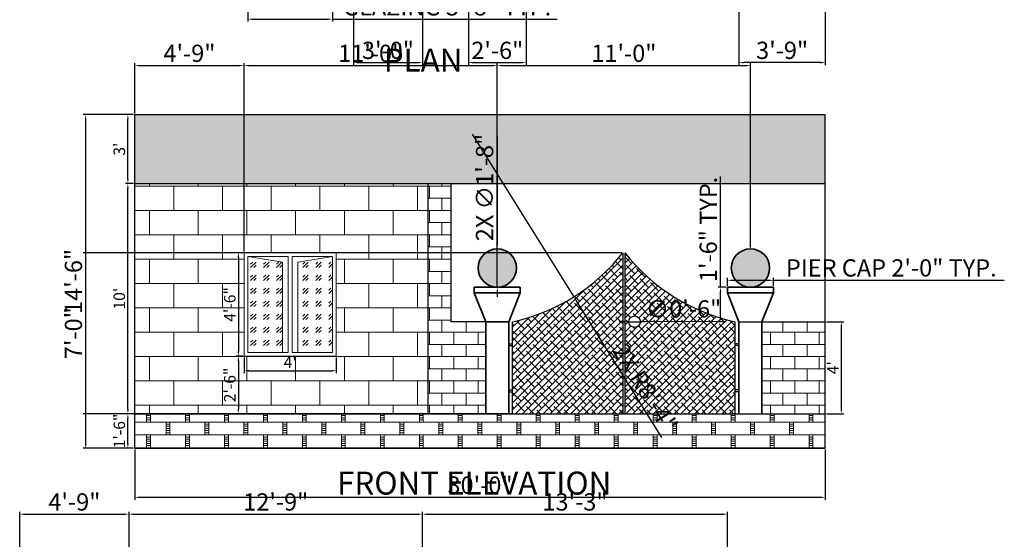
# Model space of a CAD drawing. Units: inches. Extents: x 2639 to 6021, y 292 to 2009.
# Tile 3 of 6: x 2676 to 3189, y 971 to 1243. Entities that reach past the tile are written whole.
import ezdxf

# ---------------------------------------------------------------- set-up
doc = ezdxf.new("R2010")
doc.units = ezdxf.units.IN
for name, color, linetype, lineweight in [('A-ANNO-DIMS', 2, 'Continuous', 18), ('A-ANNO-TEXT', 7, 'Continuous', 18), ('A-COLS', 7, 'Continuous', 35), ('A-DOOR-GATE', 3, 'Continuous', 25), ('A-ELEV', 7, 'Continuous', 30), ('A-ELEV-PATT', 8, 'Continuous', 13), ('A-GLAZ', 4, 'Continuous', 18), ('A-GLAZ-PATT', 9, 'Continuous', 13)]:
    doc.layers.add(name, color=color, linetype=linetype, lineweight=lineweight)
for name, color, linetype, lineweight, true_color in [('A-COLS-PATT', 251, 'Continuous', 13, 0x636466), ('A-DOOR-GATE-PATT', 251, 'Continuous', 13, 0x636466), ('A-ELEV-MASN-PATT', 30, 'Continuous', 13, 0xf26722)]:
    doc.layers.add(name, color=color, linetype=linetype, lineweight=lineweight, true_color=true_color)
doc.styles.get("Standard").update_dxf_attribs({"font": 'arial.ttf'})
doc.dimstyles.new('ISO-25', dxfattribs={"dimtxt": 9, "dimasz": 2.5, "dimexe": 1.25, "dimexo": 0.625, "dimtad": 1, "dimdec": 1, "dimlunit": 3, "dimtxsty": 'Standard', "dimcen": 2.5, "dimadec": 0, "dimazin": 0, "dimtfac": 1, "dimtdec": 1, "dimtmove": 0, "dimatfit": 3, "dimfxl": 1, "dimarcsym": 0})

# ---------------------------------------------------------------- blocks, each defined once
blk = doc.blocks.new('*D9')
at = {"layer": 'A-ANNO-DIMS', "color": 0, "lineweight": -2, "transparency": 16777216}
for p, q in [((2735.48, 1036.99), (2731.25, 1036.99)), ((2732.5, 1021.49), (2732.5, 1034.49)), ((2735.48, 1018.99), (2731.25, 1018.99))]:
    blk.add_line(p, q, dxfattribs=at)
at = {"layer": 'A-ANNO-DIMS', "color": 0, "transparency": 16777216}
for points in [[(2732.09, 1034.49), (2732.92, 1034.49), (2732.5, 1036.99)], [(2732.09, 1021.49), (2732.92, 1021.49), (2732.5, 1018.99)]]:
    blk.add_solid(points, dxfattribs=at)
at = {"layer": 'Defpoints', "color": 0, "transparency": 16777216}
for p in [(2732.5, 1036.99), (2736.11, 1036.99), (2736.11, 1018.99)]:
    blk.add_point(p, dxfattribs=at)
at = {"layer": 'A-ANNO-DIMS', "color": 0, "transparency": 16777216, "insert": (2728.81, 1027.99), "char_height": 6, "attachment_point": 5, "rotation": 90}
blk.add_mtext('1\'-6"', dxfattribs=at)
blk = doc.blocks.new('*D10')
at = {"layer": 'A-ANNO-DIMS', "color": 0, "lineweight": -2, "transparency": 16777216}
for p, q in [((2735.48, 1156.99), (2731.25, 1156.99)), ((2732.5, 1039.49), (2732.5, 1154.49)), ((2735.48, 1036.99), (2731.25, 1036.99))]:
    blk.add_line(p, q, dxfattribs=at)
at = {"layer": 'A-ANNO-DIMS', "color": 0, "transparency": 16777216}
for points in [[(2732.09, 1154.49), (2732.92, 1154.49), (2732.5, 1156.99)], [(2732.09, 1039.49), (2732.92, 1039.49), (2732.5, 1036.99)]]:
    blk.add_solid(points, dxfattribs=at)
at = {"layer": 'Defpoints', "color": 0, "transparency": 16777216}
for p in [(2732.5, 1156.99), (2736.11, 1156.99), (2736.11, 1036.99)]:
    blk.add_point(p, dxfattribs=at)
at = {"layer": 'A-ANNO-DIMS', "color": 0, "transparency": 16777216, "insert": (2728.81, 1096.99), "char_height": 6, "attachment_point": 5, "rotation": 90}
blk.add_mtext("10'", dxfattribs=at)
blk = doc.blocks.new('*D11')
at = {"layer": 'A-ANNO-DIMS', "color": 0, "lineweight": -2, "transparency": 16777216}
for p, q in [((2735.48, 1192.99), (2731.25, 1192.99)), ((2732.5, 1159.49), (2732.5, 1190.49)), ((2735.48, 1156.99), (2731.25, 1156.99))]:
    blk.add_line(p, q, dxfattribs=at)
at = {"layer": 'A-ANNO-DIMS', "color": 0, "transparency": 16777216}
for points in [[(2732.09, 1190.49), (2732.92, 1190.49), (2732.5, 1192.99)], [(2732.09, 1159.49), (2732.92, 1159.49), (2732.5, 1156.99)]]:
    blk.add_solid(points, dxfattribs=at)
at = {"layer": 'Defpoints', "color": 0, "transparency": 16777216}
for p in [(2732.5, 1192.99), (2736.11, 1192.99), (2736.11, 1156.99)]:
    blk.add_point(p, dxfattribs=at)
at = {"layer": 'A-ANNO-DIMS', "color": 0, "transparency": 16777216, "insert": (2728.81, 1174.99), "char_height": 6, "attachment_point": 5, "rotation": 90}
blk.add_mtext("3'", dxfattribs=at)
blk = doc.blocks.new('*D12')
at = {"layer": 'A-ANNO-DIMS', "color": 0, "lineweight": -2, "transparency": 16777216}
for p, q in [((2793.11, 1066.36), (2793.11, 1058.14)), ((2841.11, 1066.36), (2841.11, 1058.14)), ((2795.61, 1059.39), (2838.61, 1059.39))]:
    blk.add_line(p, q, dxfattribs=at)
at = {"layer": 'A-ANNO-DIMS', "color": 0, "transparency": 16777216}
for points in [[(2795.61, 1059.81), (2795.61, 1058.97), (2793.11, 1059.39)], [(2838.61, 1059.81), (2838.61, 1058.97), (2841.11, 1059.39)]]:
    blk.add_solid(points, dxfattribs=at)
at = {"layer": 'Defpoints', "color": 0, "transparency": 16777216}
for p in [(2793.11, 1066.99), (2841.11, 1066.99), (2841.11, 1059.39)]:
    blk.add_point(p, dxfattribs=at)
at = {"layer": 'A-ANNO-DIMS', "color": 0, "transparency": 16777216, "insert": (2817.11, 1063.02), "char_height": 6, "attachment_point": 5}
blk.add_mtext("4'", dxfattribs=at)
blk = doc.blocks.new('*D13')
at = {"layer": 'A-ANNO-DIMS', "color": 0, "lineweight": -2, "transparency": 16777216}
for p, q in [((2792.48, 1120.99), (2788.86, 1120.99)), ((2790.11, 1118.49), (2790.11, 1069.49)), ((2792.48, 1066.99), (2788.86, 1066.99))]:
    blk.add_line(p, q, dxfattribs=at)
at = {"layer": 'A-ANNO-DIMS', "color": 0, "transparency": 16777216}
for points in [[(2789.69, 1118.49), (2790.52, 1118.49), (2790.11, 1120.99)], [(2789.69, 1069.49), (2790.52, 1069.49), (2790.11, 1066.99)]]:
    blk.add_solid(points, dxfattribs=at)
at = {"layer": 'Defpoints', "color": 0, "transparency": 16777216}
for p in [(2793.11, 1120.99), (2790.11, 1066.99), (2793.11, 1066.99)]:
    blk.add_point(p, dxfattribs=at)
at = {"layer": 'A-ANNO-DIMS', "color": 0, "transparency": 16777216, "insert": (2786.42, 1093.99), "char_height": 6, "attachment_point": 5, "rotation": 90}
blk.add_mtext('4\'-6"', dxfattribs=at)
blk = doc.blocks.new('*D14')
at = {"layer": 'A-ANNO-DIMS', "color": 0, "lineweight": -2, "transparency": 16777216}
for p, q in [((2792.48, 1066.99), (2788.86, 1066.99)), ((2790.11, 1064.49), (2790.11, 1039.49)), ((2790.73, 1036.99), (2791.36, 1036.99))]:
    blk.add_line(p, q, dxfattribs=at)
at = {"layer": 'A-ANNO-DIMS', "color": 0, "transparency": 16777216}
for points in [[(2789.69, 1064.49), (2790.52, 1064.49), (2790.11, 1066.99)], [(2789.69, 1039.49), (2790.52, 1039.49), (2790.11, 1036.99)]]:
    blk.add_solid(points, dxfattribs=at)
at = {"layer": 'Defpoints', "color": 0, "transparency": 16777216}
for p in [(2793.11, 1066.99), (2790.11, 1036.99), (2790.11, 1036.99)]:
    blk.add_point(p, dxfattribs=at)
at = {"layer": 'A-ANNO-DIMS', "color": 0, "transparency": 16777216, "insert": (2786.42, 1051.99), "char_height": 6, "attachment_point": 5, "rotation": 90}
blk.add_mtext('2\'-6"', dxfattribs=at)
blk = doc.blocks.new('*D21')
at = {"layer": 'A-ANNO-DIMS', "color": 0, "lineweight": -2, "transparency": 16777216}
for p, q in [((3096.73, 1084.99), (3105.72, 1084.99)), ((3104.47, 1082.49), (3104.47, 1039.49)), ((3096.73, 1036.99), (3105.72, 1036.99))]:
    blk.add_line(p, q, dxfattribs=at)
at = {"layer": 'A-ANNO-DIMS', "color": 0, "transparency": 16777216}
for points in [[(3104.05, 1082.49), (3104.88, 1082.49), (3104.47, 1084.99)], [(3104.05, 1039.49), (3104.88, 1039.49), (3104.47, 1036.99)]]:
    blk.add_solid(points, dxfattribs=at)
at = {"layer": 'Defpoints', "color": 0, "transparency": 16777216}
for p in [(3096.11, 1084.99), (3096.11, 1036.99), (3104.47, 1036.99)]:
    blk.add_point(p, dxfattribs=at)
at = {"layer": 'A-ANNO-DIMS', "color": 0, "transparency": 16777216, "insert": (3100.84, 1060.99), "char_height": 6, "attachment_point": 5, "rotation": 90}
blk.add_mtext("4'", dxfattribs=at)
blk = doc.blocks.new('GATE-PIER-CAP')
for p, q in [((0, 18), (24, 18)), ((0, 18), (0, 15)), ((24, 15), (24, 18)), ((0, 15), (6, 0)), ((0, 15), (24, 15)), ((18, 0), (24, 15))]:
    blk.add_line(p, q)
blk = doc.blocks.new('*D32')
at = {"layer": 'A-ANNO-DIMS', "color": 0, "lineweight": -2, "transparency": 16777216}
for p, q in [((2795.11, 1248.76), (2795.11, 1241.53)), ((2839.11, 1248.76), (2839.11, 1241.53)), ((2797.61, 1242.78), (2836.61, 1242.78)), ((2839.11, 1242.78), (2956.25, 1242.78))]:
    blk.add_line(p, q, dxfattribs=at)
at = {"layer": 'A-ANNO-DIMS', "color": 0, "transparency": 16777216}
for points in [[(2797.61, 1243.2), (2797.61, 1242.37), (2795.11, 1242.78)], [(2836.61, 1243.2), (2836.61, 1242.37), (2839.11, 1242.78)]]:
    blk.add_solid(points, dxfattribs=at)
at = {"layer": 'Defpoints', "color": 0, "transparency": 16777216}
for p in [(2795.11, 1249.38), (2839.11, 1249.38), (2839.11, 1242.78)]:
    blk.add_point(p, dxfattribs=at)
at = {"layer": 'A-ANNO-DIMS', "color": 0, "transparency": 16777216, "insert": (2898.93, 1248.07), "char_height": 9, "attachment_point": 5}
blk.add_mtext('GLAZING 3\'-8" TYP.', dxfattribs=at)
blk = doc.blocks.new('*D42')
at = {"layer": 'A-ANNO-DIMS', "color": 0, "lineweight": -2, "transparency": 16777216}
for p, q in [((3045.11, 1103.61), (3045.11, 1107.84)), ((3047.61, 1106.59), (3066.61, 1106.59)), ((3069.11, 1103.61), (3069.11, 1107.84)), ((3069.11, 1106.59), (3189.45, 1106.59))]:
    blk.add_line(p, q, dxfattribs=at)
at = {"layer": 'A-ANNO-DIMS', "color": 0, "transparency": 16777216}
for points in [[(3047.61, 1107), (3047.61, 1106.17), (3045.11, 1106.59)], [(3066.61, 1107), (3066.61, 1106.17), (3069.11, 1106.59)]]:
    blk.add_solid(points, dxfattribs=at)
at = {"layer": 'Defpoints', "color": 0, "transparency": 16777216}
for p in [(3069.11, 1106.59), (3045.11, 1102.99), (3069.11, 1102.99)]:
    blk.add_point(p, dxfattribs=at)
at = {"layer": 'A-ANNO-DIMS', "color": 0, "transparency": 16777216, "insert": (3130.53, 1111.87), "char_height": 9, "attachment_point": 5}
blk.add_mtext('PIER CAP 2\'-0" TYP.', dxfattribs=at)
blk = doc.blocks.new('*D43')
at = {"layer": 'A-ANNO-DIMS', "color": 0, "lineweight": -2, "transparency": 16777216}
for p, q in [((3041.51, 1102.99), (3041.51, 1160.75)), ((3044.48, 1102.99), (3040.26, 1102.99)), ((3041.51, 1087.49), (3041.51, 1100.49)), ((3044.48, 1084.99), (3040.26, 1084.99))]:
    blk.add_line(p, q, dxfattribs=at)
at = {"layer": 'A-ANNO-DIMS', "color": 0, "transparency": 16777216}
for points in [[(3041.09, 1100.49), (3041.92, 1100.49), (3041.51, 1102.99)], [(3041.09, 1087.49), (3041.92, 1087.49), (3041.51, 1084.99)]]:
    blk.add_solid(points, dxfattribs=at)
at = {"layer": 'Defpoints', "color": 0, "transparency": 16777216}
for p in [(3041.51, 1102.99), (3045.11, 1102.99), (3045.11, 1084.99)]:
    blk.add_point(p, dxfattribs=at)
at = {"layer": 'A-ANNO-DIMS', "color": 0, "transparency": 16777216, "insert": (3036.29, 1133.12), "char_height": 9, "attachment_point": 5, "rotation": 90}
blk.add_mtext('1\'-6" TYP.', dxfattribs=at)
blk = doc.blocks.new('*D54')
at = {"layer": 'A-ANNO-DIMS', "color": 0, "lineweight": -2, "transparency": 16777216}
for p, q in [((2850.11, 1569.76), (2850.11, 1218.88)), ((2886.11, 1569.76), (2886.11, 1218.88)), ((2852.61, 1220.13), (2883.61, 1220.13))]:
    blk.add_line(p, q, dxfattribs=at)
at = {"layer": 'A-ANNO-DIMS', "color": 0, "transparency": 16777216}
for points in [[(2852.61, 1220.55), (2852.61, 1219.72), (2850.11, 1220.13)], [(2883.61, 1220.55), (2883.61, 1219.72), (2886.11, 1220.13)]]:
    blk.add_solid(points, dxfattribs=at)
at = {"layer": 'Defpoints', "color": 0, "transparency": 16777216}
for p in [(2850.11, 1570.38), (2886.11, 1570.38), (2886.11, 1220.13)]:
    blk.add_point(p, dxfattribs=at)
at = {"layer": 'A-ANNO-DIMS', "color": 0, "transparency": 16777216, "insert": (2868.11, 1225.36), "char_height": 9, "attachment_point": 5}
blk.add_mtext('3\'-0"', dxfattribs=at)
blk = doc.blocks.new('*D55')
at = {"layer": 'A-ANNO-DIMS', "color": 0, "lineweight": -2, "transparency": 16777216}
for p, q in [((2910.11, 1617.76), (2910.11, 1218.88)), ((2940.11, 1617.76), (2940.11, 1218.88)), ((2912.61, 1220.13), (2937.61, 1220.13))]:
    blk.add_line(p, q, dxfattribs=at)
at = {"layer": 'A-ANNO-DIMS', "color": 0, "transparency": 16777216}
for points in [[(2912.61, 1220.55), (2912.61, 1219.72), (2910.11, 1220.13)], [(2937.61, 1220.55), (2937.61, 1219.72), (2940.11, 1220.13)]]:
    blk.add_solid(points, dxfattribs=at)
at = {"layer": 'Defpoints', "color": 0, "transparency": 16777216}
for p in [(2910.11, 1618.38), (2940.11, 1618.38), (2940.11, 1220.13)]:
    blk.add_point(p, dxfattribs=at)
at = {"layer": 'A-ANNO-DIMS', "color": 0, "transparency": 16777216, "insert": (2925.11, 1225.35), "char_height": 9, "attachment_point": 5}
blk.add_mtext('2\'-6"', dxfattribs=at)
blk = doc.blocks.new('*D59')
at = {"layer": 'A-ANNO-DIMS', "color": 0, "lineweight": -2, "transparency": 16777216}
for p, q in [((3051.11, 1248.76), (3051.11, 1218.88)), ((3096.11, 1248.76), (3096.11, 1218.88)), ((3093.61, 1220.13), (3053.61, 1220.13))]:
    blk.add_line(p, q, dxfattribs=at)
at = {"layer": 'A-ANNO-DIMS', "color": 0, "transparency": 16777216}
for points in [[(3053.61, 1220.55), (3053.61, 1219.72), (3051.11, 1220.13)], [(3093.61, 1220.55), (3093.61, 1219.72), (3096.11, 1220.13)]]:
    blk.add_solid(points, dxfattribs=at)
at = {"layer": 'Defpoints', "color": 0, "transparency": 16777216}
for p in [(3051.11, 1249.38), (3096.11, 1249.38), (3051.11, 1220.13)]:
    blk.add_point(p, dxfattribs=at)
at = {"layer": 'A-ANNO-DIMS', "color": 0, "transparency": 16777216, "insert": (3073.61, 1225.36), "char_height": 9, "attachment_point": 5}
blk.add_mtext('3\'-9"', dxfattribs=at)
blk = doc.blocks.new('*D72')
at = {"layer": 'A-ANNO-DIMS', "color": 0, "lineweight": -2, "transparency": 16777216}
for p, q in [((2925.11, 1123.61), (2925.11, 1219.84)), ((2927.61, 1218.59), (3054.61, 1218.59)), ((3057.11, 1123.61), (3057.11, 1219.84))]:
    blk.add_line(p, q, dxfattribs=at)
at = {"layer": 'A-ANNO-DIMS', "color": 0, "transparency": 16777216}
for points in [[(2927.61, 1219), (2927.61, 1218.17), (2925.11, 1218.59)], [(3054.61, 1219), (3054.61, 1218.17), (3057.11, 1218.59)]]:
    blk.add_solid(points, dxfattribs=at)
at = {"layer": 'Defpoints', "color": 0, "transparency": 16777216}
for p in [(3057.11, 1218.59), (2925.11, 1122.99), (3057.11, 1122.99)]:
    blk.add_point(p, dxfattribs=at)
at = {"layer": 'A-ANNO-DIMS', "color": 0, "transparency": 16777216, "insert": (2991.11, 1223.81), "char_height": 9, "attachment_point": 5}
blk.add_mtext('11\'-0"', dxfattribs=at)
blk = doc.blocks.new('*D73')
at = {"layer": 'A-ANNO-DIMS', "color": 0, "lineweight": -2, "transparency": 16777216}
for p, q in [((2989.98, 1120.99), (2709.26, 1120.99)), ((2710.51, 1039.49), (2710.51, 1118.49)), ((2932.48, 1036.99), (2709.26, 1036.99))]:
    blk.add_line(p, q, dxfattribs=at)
at = {"layer": 'A-ANNO-DIMS', "color": 0, "transparency": 16777216}
for points in [[(2710.09, 1118.49), (2710.92, 1118.49), (2710.51, 1120.99)], [(2710.09, 1039.49), (2710.92, 1039.49), (2710.51, 1036.99)]]:
    blk.add_solid(points, dxfattribs=at)
at = {"layer": 'Defpoints', "color": 0, "transparency": 16777216}
for p in [(2710.51, 1120.99), (2990.61, 1120.99), (2933.11, 1036.99)]:
    blk.add_point(p, dxfattribs=at)
at = {"layer": 'A-ANNO-DIMS', "color": 0, "transparency": 16777216, "insert": (2705.29, 1078.99), "char_height": 9, "attachment_point": 5, "rotation": 90}
blk.add_mtext('7\'-0"', dxfattribs=at)
blk = doc.blocks.new('*D74')
at = {"layer": 'A-ANNO-DIMS', "color": 0, "lineweight": -2, "transparency": 16777216}
for p, q in [((2736.11, 1018.36), (2736.11, 992.14)), ((3096.11, 1018.36), (3096.11, 992.14)), ((2738.61, 993.39), (3093.61, 993.39))]:
    blk.add_line(p, q, dxfattribs=at)
at = {"layer": 'A-ANNO-DIMS', "color": 0, "transparency": 16777216}
for points in [[(2738.61, 993.8), (2738.61, 992.97), (2736.11, 993.39)], [(3093.61, 993.8), (3093.61, 992.97), (3096.11, 993.39)]]:
    blk.add_solid(points, dxfattribs=at)
at = {"layer": 'Defpoints', "color": 0, "transparency": 16777216}
for p in [(2736.11, 1018.99), (3096.11, 1018.99), (3096.11, 993.39)]:
    blk.add_point(p, dxfattribs=at)
at = {"layer": 'A-ANNO-DIMS', "color": 0, "transparency": 16777216, "insert": (2916.11, 998.61), "char_height": 9, "attachment_point": 5}
blk.add_mtext('30\'-0"', dxfattribs=at)
blk = doc.blocks.new('*D75')
at = {"layer": 'A-ANNO-DIMS', "color": 0, "lineweight": -2, "transparency": 16777216}
for p, q in [((2735.48, 1192.99), (2709.26, 1192.99)), ((2710.51, 1021.49), (2710.51, 1190.49)), ((2735.48, 1018.99), (2709.26, 1018.99))]:
    blk.add_line(p, q, dxfattribs=at)
at = {"layer": 'A-ANNO-DIMS', "color": 0, "transparency": 16777216}
for points in [[(2710.09, 1190.49), (2710.92, 1190.49), (2710.51, 1192.99)], [(2710.09, 1021.49), (2710.92, 1021.49), (2710.51, 1018.99)]]:
    blk.add_solid(points, dxfattribs=at)
at = {"layer": 'Defpoints', "color": 0, "transparency": 16777216}
for p in [(2710.51, 1192.99), (2736.11, 1192.99), (2736.11, 1018.99)]:
    blk.add_point(p, dxfattribs=at)
at = {"layer": 'A-ANNO-DIMS', "color": 0, "transparency": 16777216, "insert": (2705.29, 1105.99), "char_height": 9, "attachment_point": 5, "rotation": 90}
blk.add_mtext('14\'-6"', dxfattribs=at)
blk = doc.blocks.new('*D76')
at = {"layer": 'A-ANNO-DIMS', "color": 0, "lineweight": -2, "transparency": 16777216}
for p, q in [((2736.11, 1193.61), (2736.11, 1219.84)), ((2738.61, 1218.59), (2790.61, 1218.59)), ((2793.11, 1121.61), (2793.11, 1219.84))]:
    blk.add_line(p, q, dxfattribs=at)
at = {"layer": 'A-ANNO-DIMS', "color": 0, "transparency": 16777216}
for points in [[(2738.61, 1219), (2738.61, 1218.17), (2736.11, 1218.59)], [(2790.61, 1219), (2790.61, 1218.17), (2793.11, 1218.59)]]:
    blk.add_solid(points, dxfattribs=at)
at = {"layer": 'Defpoints', "color": 0, "transparency": 16777216}
for p in [(2793.11, 1218.59), (2736.11, 1192.99), (2793.11, 1120.99)]:
    blk.add_point(p, dxfattribs=at)
at = {"layer": 'A-ANNO-DIMS', "color": 0, "transparency": 16777216, "insert": (2764.61, 1223.81), "char_height": 9, "attachment_point": 5}
blk.add_mtext('4\'-9"', dxfattribs=at)
blk = doc.blocks.new('*D77')
at = {"layer": 'A-ANNO-DIMS', "color": 0, "lineweight": -2, "transparency": 16777216}
for p, q in [((2793.11, 1121.61), (2793.11, 1219.84)), ((2795.61, 1218.59), (2922.61, 1218.59)), ((2925.11, 1113.61), (2925.11, 1219.84))]:
    blk.add_line(p, q, dxfattribs=at)
at = {"layer": 'A-ANNO-DIMS', "color": 0, "transparency": 16777216}
for points in [[(2795.61, 1219), (2795.61, 1218.17), (2793.11, 1218.59)], [(2922.61, 1219), (2922.61, 1218.17), (2925.11, 1218.59)]]:
    blk.add_solid(points, dxfattribs=at)
at = {"layer": 'Defpoints', "color": 0, "transparency": 16777216}
for p in [(2925.11, 1218.59), (2793.11, 1120.99), (2925.11, 1112.99)]:
    blk.add_point(p, dxfattribs=at)
at = {"layer": 'A-ANNO-DIMS', "color": 0, "transparency": 16777216, "insert": (2859.11, 1223.81), "char_height": 9, "attachment_point": 5}
blk.add_mtext('11\'-0"', dxfattribs=at)
blk = doc.blocks.new('*D88')
at = {"layer": 'A-ANNO-DIMS', "color": 0, "lineweight": -2, "transparency": 16777216}
for p, q in [((2676.11, 959.61), (2676.11, 985.84)), ((2733.11, 887.61), (2733.11, 985.84)), ((2678.61, 984.59), (2730.61, 984.59))]:
    blk.add_line(p, q, dxfattribs=at)
at = {"layer": 'A-ANNO-DIMS', "color": 0, "transparency": 16777216}
for points in [[(2678.61, 985), (2678.61, 984.17), (2676.11, 984.59)], [(2730.61, 985), (2730.61, 984.17), (2733.11, 984.59)]]:
    blk.add_solid(points, dxfattribs=at)
at = {"layer": 'Defpoints', "color": 0, "transparency": 16777216}
for p in [(2733.11, 984.59), (2676.11, 958.99), (2733.11, 886.99)]:
    blk.add_point(p, dxfattribs=at)
at = {"layer": 'A-ANNO-DIMS', "color": 0, "transparency": 16777216, "insert": (2704.61, 989.81), "char_height": 9, "attachment_point": 5}
blk.add_mtext('4\'-9"', dxfattribs=at)
blk = doc.blocks.new('*D89')
at = {"layer": 'A-ANNO-DIMS', "color": 0, "lineweight": -2, "transparency": 16777216}
for p, q in [((2733.11, 887.61), (2733.11, 985.84)), ((2886.11, 887.61), (2886.11, 985.84)), ((2735.61, 984.59), (2883.61, 984.59))]:
    blk.add_line(p, q, dxfattribs=at)
at = {"layer": 'A-ANNO-DIMS', "color": 0, "transparency": 16777216}
for points in [[(2735.61, 985), (2735.61, 984.17), (2733.11, 984.59)], [(2883.61, 985), (2883.61, 984.17), (2886.11, 984.59)]]:
    blk.add_solid(points, dxfattribs=at)
at = {"layer": 'Defpoints', "color": 0, "transparency": 16777216}
for p in [(2886.11, 984.59), (2733.11, 886.99), (2886.11, 886.99)]:
    blk.add_point(p, dxfattribs=at)
at = {"layer": 'A-ANNO-DIMS', "color": 0, "transparency": 16777216, "insert": (2809.61, 989.81), "char_height": 9, "attachment_point": 5}
blk.add_mtext('12\'-9"', dxfattribs=at)
blk = doc.blocks.new('*D90')
at = {"layer": 'A-ANNO-DIMS', "color": 0, "lineweight": -2, "transparency": 16777216}
for p, q in [((2886.11, 887.61), (2886.11, 985.84)), ((3045.11, 887.61), (3045.11, 985.84)), ((2888.61, 984.59), (3042.61, 984.59))]:
    blk.add_line(p, q, dxfattribs=at)
at = {"layer": 'A-ANNO-DIMS', "color": 0, "transparency": 16777216}
for points in [[(2888.61, 985), (2888.61, 984.17), (2886.11, 984.59)], [(3042.61, 985), (3042.61, 984.17), (3045.11, 984.59)]]:
    blk.add_solid(points, dxfattribs=at)
at = {"layer": 'Defpoints', "color": 0, "transparency": 16777216}
for p in [(3045.11, 984.59), (2886.11, 886.99), (3045.11, 886.99)]:
    blk.add_point(p, dxfattribs=at)
at = {"layer": 'A-ANNO-DIMS', "color": 0, "transparency": 16777216, "insert": (2965.61, 989.81), "char_height": 9, "attachment_point": 5}
blk.add_mtext('13\'-3"', dxfattribs=at)
blk = doc.blocks.new('*D114')
at = {"layer": 'A-ANNO-DIMS', "color": 0, "lineweight": -2, "transparency": 16777216}
for p, q in [((2911.93, 1182.73), (2965, 1097.96)), ((3010.98, 1024.52), (2966.33, 1095.84))]:
    blk.add_line(p, q, dxfattribs=at)
at = {"layer": 'A-ANNO-DIMS', "color": 0, "transparency": 16777216}
blk.add_solid([(2966.68, 1096.06), (2965.98, 1095.62), (2965, 1097.96)], dxfattribs=at)
at = {"layer": 'Defpoints', "color": 0, "transparency": 16777216}
for p in [(2911.93, 1182.73), (2965, 1097.96)]:
    blk.add_point(p, dxfattribs=at)
at = {"layer": 'A-ANNO-DIMS', "color": 0, "transparency": 16777216, "insert": (3001.27, 1049.87), "char_height": 9, "attachment_point": 5, "rotation": 302.05}
blk.add_mtext('2X R8\'-4"', dxfattribs=at)
blk = doc.blocks.new('*D115')
at = {"layer": 'A-ANNO-DIMS', "color": 0, "lineweight": -2, "transparency": 16777216}
for p, q in [((2925.13, 1181.97), (2925.11, 1125.49)), ((2925.1, 1102.99), (2925.11, 1122.99)), ((2925.1, 1100.49), (2925.1, 1097.99))]:
    blk.add_line(p, q, dxfattribs=at)
at = {"layer": 'A-ANNO-DIMS', "color": 0, "transparency": 16777216}
for points in [[(2924.69, 1125.49), (2925.53, 1125.49), (2925.11, 1122.99)], [(2924.69, 1100.49), (2925.52, 1100.49), (2925.1, 1102.99)]]:
    blk.add_solid(points, dxfattribs=at)
at = {"layer": 'Defpoints', "color": 0, "transparency": 16777216}
for p in [(2925.11, 1122.99), (2925.1, 1102.99)]:
    blk.add_point(p, dxfattribs=at)
at = {"layer": 'A-ANNO-DIMS', "color": 0, "transparency": 16777216, "insert": (2919.65, 1154.98), "char_height": 9, "attachment_point": 5, "rotation": 89.9845}
blk.add_mtext('2X ∅1\'-8"', dxfattribs=at)
blk = doc.blocks.new('*D116')
at = {"layer": 'A-ANNO-DIMS', "color": 0, "lineweight": -2, "transparency": 16777216}
for p, q in [((2991.19, 1084.98), (2988.69, 1084.98)), ((2993.69, 1084.98), (2999.69, 1084.99)), ((3039.66, 1085.03), (3002.19, 1084.99))]:
    blk.add_line(p, q, dxfattribs=at)
at = {"layer": 'A-ANNO-DIMS', "color": 0, "transparency": 16777216}
for points in [[(2991.19, 1085.4), (2991.19, 1084.56), (2993.69, 1084.98)], [(3002.19, 1085.41), (3002.19, 1084.58), (2999.69, 1084.99)]]:
    blk.add_solid(points, dxfattribs=at)
at = {"layer": 'Defpoints', "color": 0, "transparency": 16777216}
for p in [(2993.69, 1084.98), (2999.69, 1084.99)]:
    blk.add_point(p, dxfattribs=at)
at = {"layer": 'A-ANNO-DIMS', "color": 0, "transparency": 16777216, "insert": (3022.17, 1090.49), "char_height": 9, "attachment_point": 5, "rotation": 0.0598}
blk.add_mtext('∅0\'-6"', dxfattribs=at)

msp = doc.modelspace()

# ---------------------------------------------------------------- hatches: boundary and pattern name
at = {"layer": 'A-COLS-PATT'}
h = msp.add_hatch(color=256, dxfattribs=at)
h.dxf.hatch_style = 1
h.set_gradient(color1=(205, 105, 40), color2=(255, 255, 0), name='SPHERICAL')
h.paths.add_polyline_path([(2915.11, 1112.99, 1), (2935.11, 1112.99, 1)])
h = msp.add_hatch(color=256, dxfattribs=at)
h.dxf.hatch_style = 1
h.set_gradient(color1=(205, 105, 40), color2=(255, 255, 0), name='SPHERICAL')
h.paths.add_polyline_path([(3067.11, 1112.99, 1), (3047.11, 1112.99, 1)])
at = {"layer": 'A-DOOR-GATE-PATT'}
h = msp.add_hatch(dxfattribs=at)
h.set_pattern_fill('ANSI38', color=256, scale=0.8)
h.set_pattern_definition([(45, (-1561.5478, 0), (-1.7960512, 1.7960512), []), (135, (-1561.5478, 0), (-5.3881537, 1.7960512), [6.35, -3.81])])
h.paths.add_polyline_path([(2990.61, 1036.99), (2990.61, 1120.99, -0.174766), (2933.11, 1084.99), (2933.11, 1036.99)])
h.paths.add_polyline_path([(3049.11, 1036.99), (3049.11, 1084.99, -0.174766), (2991.61, 1120.99), (2991.61, 1036.99)])
h.paths.add_polyline_path([(2993.69, 1084.99, -1), (2999.69, 1084.99, -1)], flags=16)
at = {"layer": 'A-ELEV-MASN-PATT'}
h = msp.add_hatch(dxfattribs=at)
h.set_pattern_fill('BRICK', color=256, scale=2)
h.set_pattern_definition([(0, (-1561.548, 0), (0, 12.7), []), (90, (-1561.548, 0), (-25.4, 2e-15), [12.7, -12.7]), (90, (-1548.848, 0), (-25.4, 2e-15), [-12.7, 12.7])])
h.paths.add_polyline_path([(2889.11, 1156.99), (2736.11, 1156.99), (2736.11, 1036.99), (2889.11, 1036.99)])
h.paths.add_polyline_path([(2841.11, 1066.99), (2793.11, 1066.99), (2793.11, 1120.99), (2841.11, 1120.99)], flags=16)
h.paths.add_polyline_path([(2839.11, 1068.99), (2818.11, 1068.99), (2818.11, 1118.99), (2839.11, 1118.99)], flags=0)
h.paths.add_polyline_path([(2816.11, 1068.99), (2795.11, 1068.99), (2795.11, 1118.99), (2816.11, 1118.99)], flags=0)
h = msp.add_hatch(dxfattribs=at)
h.set_pattern_fill('BRICK', color=256)
h.set_pattern_definition([(0, (-1561.548, 0), (0, 6.35), []), (90, (-1561.548, 0), (-12.7, 8e-16), [6.35, -6.35]), (90, (-1555.198, 0), (-12.7, 8e-16), [-6.35, 6.35])])
h.paths.add_polyline_path([(2889.11, 1036.99), (2919.11, 1036.99), (2919.11, 1084.99), (2901.11, 1084.99), (2901.11, 1156.99), (2889.11, 1156.99)])
h.paths.add_polyline_path([(3063.11, 1036.99), (3096.11, 1036.99), (3096.11, 1084.99), (3063.11, 1084.99)])
at = {"layer": 'A-ELEV-PATT'}
h = msp.add_hatch(dxfattribs=at)
h.set_pattern_fill('STARS', color=256, scale=0.8)
h.set_pattern_definition([(0, (-1561.548, 0), (0, 4.399409), [2.54, -2.54]), (60, (-1561.548, 0), (-3.81, 2.1997045), [2.54, -2.54]), (120, (-1560.278, 2.1997), (-3.81, -2.1997045), [2.54, -2.54])])
h.paths.add_polyline_path([(2736.11, 1192.99), (2736.11, 1156.99), (3096.11, 1156.99), (3096.11, 1192.99)])
h = msp.add_hatch(dxfattribs=at)
h.set_pattern_fill('BRSTONE', color=256, scale=0.8)
h.set_pattern_definition([(0, (-1561.548, 0), (0, 6.7056), []), (90, (-1543.26, 0), (-10.16, 6.7056), [6.7056, -6.7056]), (90, (-1545.292, 0), (-10.16, 6.7056), [6.7056, -6.7056]), (0, (-1543.26, 1.1176), (10.16, 6.7056), [-18.288, 2.032]), (0, (-1543.26, 2.235), (10.16, 6.7056), [-18.288, 2.032]), (0, (-1543.26, 3.353), (10.16, 6.7056), [-18.288, 2.032]), (0, (-1543.26, 4.4704), (10.16, 6.7056), [-18.288, 2.032]), (0, (-1543.26, 5.588), (10.16, 6.7056), [-18.288, 2.032])])
h.paths.add_polyline_path([(2736.11, 1036.99), (2736.11, 1018.99), (3096.11, 1018.99), (3096.11, 1036.99)])
at = {"layer": 'A-GLAZ-PATT'}
h = msp.add_hatch(dxfattribs=at)
h.set_pattern_fill('GOST_GLASS', color=256, scale=0.8)
h.set_pattern_definition([(45, (-1561.548, 0), (6.788225, 0), [4, -5.6]), (45, (-1559.851, 0), (6.788225, 0), [1.6, -8]), (45, (-1561.548, 1.697), (6.788225, 0), [1.6, -8])])
h.paths.add_polyline_path([(2813.11, 1115.99), (2795.11, 1118.99), (2795.11, 1068.99), (2813.11, 1068.99)])
h.paths.add_polyline_path([(2821.11, 1068.99), (2839.11, 1068.99), (2839.11, 1118.99), (2821.11, 1115.99)])

# ---------------------------------------------------------------- linework, layer by layer
at = {"layer": 'A-COLS'}
for p, q in [((2919.11, 1036.99), (2919.11, 1084.99)), ((2919.11, 1084.99), (2931.11, 1084.99)), ((2931.11, 1036.99), (2931.11, 1084.99)), ((3051.11, 1036.99), (3051.11, 1084.99)), ((3063.11, 1036.99), (3063.11, 1084.99))]:
    msp.add_line(p, q, dxfattribs=at)
for centre in [(2925.11, 1112.99), (3057.11, 1112.99)]:
    msp.add_circle(centre, 10, dxfattribs=at)
at = {"layer": 'A-DOOR-GATE'}
for p, q in [((2990.61, 1120.99), (2990.61, 1036.99)), ((2991.61, 1120.99), (2991.61, 1036.99)), ((2933.11, 1036.99), (2933.11, 1084.99)), ((3049.11, 1036.99), (3049.11, 1084.99)), ((2931.11, 1073.49), (2933.11, 1073.49)), ((3051.11, 1073.49), (3049.11, 1073.49)), ((2931.11, 1072.49), (2933.11, 1072.49)), ((3051.11, 1072.49), (3049.11, 1072.49)), ((2931.11, 1049.49), (2933.11, 1049.49)), ((2931.11, 1048.49), (2933.11, 1048.49)), ((3051.11, 1049.49), (3049.11, 1049.49)), ((3051.11, 1048.49), (3049.11, 1048.49))]:
    msp.add_line(p, q, dxfattribs=at)
msp.add_circle((2996.69, 1084.99), 3, dxfattribs=at)
for centre, start, end in [((2911.93, 1182.73), 282.2237, 321.8766), ((3070.28, 1182.73), 218.1234, 257.7763)]:
    msp.add_arc(centre, 100.01, start, end, dxfattribs=at)
at = {"layer": 'A-ELEV'}
for p, q in [((2736.11, 1018.99), (2736.11, 1192.99)), ((2736.11, 1192.99), (3096.11, 1192.99)), ((3096.11, 1018.99), (3096.11, 1192.99)), ((2736.11, 1156.99), (3096.11, 1156.99)), ((2889.11, 1036.99), (2889.11, 1156.99)), ((2901.11, 1084.99), (2901.11, 1156.99)), ((2919.11, 1084.99), (2901.11, 1084.99)), ((3051.11, 1084.99), (3096.11, 1084.99)), ((2736.11, 1036.99), (3096.11, 1036.99)), ((2736.11, 1018.99), (3096.11, 1018.99))]:
    msp.add_line(p, q, dxfattribs=at)
at = {"layer": 'A-GLAZ'}
for p, q in [((2793.11, 1066.99), (2793.11, 1120.99)), ((2793.11, 1120.99), (2841.11, 1120.99)), ((2841.11, 1066.99), (2841.11, 1120.99)), ((2795.11, 1068.99), (2795.11, 1118.99)), ((2795.11, 1118.99), (2816.11, 1118.99)), ((2795.11, 1118.99), (2813.11, 1115.99)), ((2813.11, 1115.99), (2813.11, 1068.99)), ((2816.11, 1118.99), (2816.11, 1068.99)), ((2818.11, 1118.99), (2818.11, 1068.99)), ((2818.11, 1118.99), (2839.11, 1118.99)), ((2821.11, 1115.99), (2839.11, 1118.99)), ((2821.11, 1115.99), (2821.11, 1068.99)), ((2839.11, 1068.99), (2839.11, 1118.99)), ((2795.11, 1068.99), (2816.11, 1068.99)), ((2818.11, 1068.99), (2839.11, 1068.99)), ((2793.11, 1066.99), (2841.11, 1066.99))]:
    msp.add_line(p, q, dxfattribs=at)

# ---------------------------------------------------------------- block references
at = {"layer": 'A-COLS'}
for p in [(2913.11, 1084.99), (3045.11, 1084.99)]:
    msp.add_blockref('GATE-PIER-CAP', p, dxfattribs=at)

# ---------------------------------------------------------------- texts
at = {"layer": 'A-ANNO-TEXT', "char_height": 12, "attachment_point": 1}
for s, insert in [('{\\fTimes New Roman|b0|i0|c0|p18;PLAN}', (2865.91, 1227.42)), ('{\\fTimes New Roman|b0|i0|c0|p18;FRONT ELEVATION}', (2841.56, 1006.81))]:
    msp.add_mtext_dynamic_manual_height_columns(s, width=172.2916, gutter_width=12.5, heights=[0], dxfattribs=dict(at, insert=insert))

# ---------------------------------------------------------------- dimensions: what is measured, and where the dimension line sits
at = {"layer": 'A-ANNO-DIMS'}
for base, p1, p2, override, picture, middle in [((2940.11, 1220.13), (2910.11, 1618.38), (2940.11, 1618.38), {"dimdec": 1, "dimlfac": 1, "dimrnd": 0, "dimzin": 1, "dimdsep": 46, "dimlunit": 4, "dimfrac": 2}, '*D55', (2925.11, 1225.35)), ((2886.11, 1220.13), (2850.11, 1570.38), (2886.11, 1570.38), {"dimdec": 1, "dimlfac": 1, "dimrnd": 0, "dimzin": 1, "dimdsep": 46, "dimlunit": 4, "dimfrac": 2}, '*D54', (2868.11, 1225.36)), ((3051.11, 1220.13), (3096.11, 1249.38), (3051.11, 1249.38), {"dimdec": 1, "dimlfac": 1, "dimrnd": 0, "dimzin": 1, "dimdsep": 46, "dimlunit": 4, "dimfrac": 2}, '*D59', (3073.61, 1225.36)), ((2793.11, 1218.59), (2736.11, 1192.99), (2793.11, 1120.99), {"dimdec": 1, "dimlfac": 1, "dimrnd": 0, "dimzin": 1, "dimdsep": 46, "dimlunit": 4, "dimfrac": 2}, '*D76', (2764.61, 1223.81)), ((2925.11, 1218.59), (2793.11, 1120.99), (2925.11, 1112.99), {"dimdec": 1, "dimlfac": 1, "dimrnd": 0, "dimzin": 1, "dimdsep": 46, "dimlunit": 4, "dimfrac": 2}, '*D77', (2859.11, 1223.81)), ((3057.11, 1218.59), (2925.11, 1122.99), (3057.11, 1122.99), {"dimdec": 1, "dimlfac": 1, "dimrnd": 0, "dimzin": 1, "dimdsep": 46, "dimlunit": 4, "dimfrac": 2}, '*D72', (2991.11, 1223.81)), ((2841.11, 1059.39), (2793.11, 1066.99), (2841.11, 1066.99), {"dimtxt": 6, "dimclrd": 0, "dimclre": 0, "dimclrt": 0}, '*D12', (2817.11, 1063.02)), ((3096.11, 993.39), (2736.11, 1018.99), (3096.11, 1018.99), {"dimdec": 1, "dimlfac": 1, "dimrnd": 0, "dimzin": 1, "dimdsep": 46, "dimlunit": 4, "dimfrac": 2}, '*D74', (2916.11, 998.61)), ((2733.11, 984.59), (2676.11, 958.99), (2733.11, 886.99), {"dimdec": 1, "dimlfac": 1, "dimrnd": 0, "dimzin": 1, "dimdsep": 46, "dimlunit": 4, "dimfrac": 2}, '*D88', (2704.61, 989.81)), ((2886.11, 984.59), (2733.11, 886.99), (2886.11, 886.99), {"dimdec": 1, "dimlfac": 1, "dimrnd": 0, "dimzin": 1, "dimdsep": 46, "dimlunit": 4, "dimfrac": 2}, '*D89', (2809.61, 989.81)), ((3045.11, 984.59), (2886.11, 886.99), (3045.11, 886.99), {"dimdec": 1, "dimlfac": 1, "dimrnd": 0, "dimzin": 1, "dimdsep": 46, "dimlunit": 4, "dimfrac": 2}, '*D90', (2965.61, 989.81))]:
    dim = msp.add_linear_dim(base=base, p1=p1, p2=p2, dimstyle='ISO-25', override=override, dxfattribs=at)
    dim.commit()
    dim.dimension.update_dxf_attribs({"geometry": picture, "text_midpoint": middle})
for base, p1, p2, text, picture, middle in [((2839.11, 1242.78), (2795.11, 1249.38), (2839.11, 1249.38), 'GLAZING <> TYP.', '*D32', (2898.93, 1248.07)), ((3069.11, 1106.59), (3045.11, 1102.99), (3069.11, 1102.99), 'PIER CAP <> TYP.', '*D42', (3130.53, 1111.87))]:
    dim = msp.add_linear_dim(base=base, p1=p1, p2=p2, text=text, dimstyle='ISO-25', override={"dimdec": 1, "dimlfac": 1, "dimrnd": 0, "dimzin": 1, "dimdsep": 46, "dimlunit": 4, "dimfrac": 2}, dxfattribs=at)
    dim.commit()
    dim.dimension.update_dxf_attribs({"geometry": picture, "text_midpoint": middle})
for base, p1, p2, override, picture, middle in [((2710.51, 1192.99), (2736.11, 1018.99), (2736.11, 1192.99), {"dimdec": 1, "dimlfac": 1, "dimrnd": 0, "dimzin": 1, "dimdsep": 46, "dimlunit": 4, "dimfrac": 2}, '*D75', (2705.29, 1105.99)), ((2732.5, 1192.99), (2736.11, 1156.99), (2736.11, 1192.99), {"dimtxt": 6, "dimclrd": 0, "dimclre": 0, "dimclrt": 0, "dimtmove": 1}, '*D11', (2728.81, 1174.99)), ((2732.5, 1156.99), (2736.11, 1036.99), (2736.11, 1156.99), {"dimtxt": 6, "dimclrd": 0, "dimclre": 0, "dimclrt": 0, "dimtmove": 1}, '*D10', (2728.81, 1096.99)), ((2710.51, 1120.99), (2933.11, 1036.99), (2990.61, 1120.99), {"dimdec": 1, "dimlfac": 1, "dimrnd": 0, "dimzin": 1, "dimdsep": 46, "dimlunit": 4, "dimfrac": 2}, '*D73', (2705.29, 1078.99)), ((2790.11, 1066.99), (2793.11, 1120.99), (2793.11, 1066.99), {"dimtxt": 6, "dimclrd": 0, "dimclre": 0, "dimclrt": 0}, '*D13', (2786.42, 1093.99)), ((3104.47, 1036.99), (3096.11, 1084.99), (3096.11, 1036.99), {"dimtxt": 6, "dimclrd": 0, "dimclre": 0, "dimclrt": 0}, '*D21', (3100.84, 1060.99)), ((2790.11, 1036.99), (2793.11, 1066.99), (2790.11, 1036.99), {"dimtxt": 6, "dimclrd": 0, "dimclre": 0, "dimclrt": 0, "dimtmove": 1}, '*D14', (2786.42, 1051.99)), ((2732.5, 1036.99), (2736.11, 1018.99), (2736.11, 1036.99), {"dimtxt": 6, "dimclrd": 0, "dimclre": 0, "dimclrt": 0}, '*D9', (2728.81, 1027.99))]:
    dim = msp.add_linear_dim(base=base, p1=p1, p2=p2, angle=90, dimstyle='ISO-25', override=override, dxfattribs=at)
    dim.commit()
    dim.dimension.update_dxf_attribs({"geometry": picture, "text_midpoint": middle})
dim = msp.add_diameter_dim_2p(p1=(2925.1, 1102.99), p2=(2925.11, 1122.99), text='2X <>', dimstyle='ISO-25', override={"dimdec": 1, "dimlfac": 1, "dimrnd": 0, "dimzin": 1, "dimdsep": 46, "dimlunit": 4, "dimfrac": 2}, dxfattribs=at)
dim.commit()
dim.dimension.update_dxf_attribs({"geometry": '*D115', "text_midpoint": (2925.12, 1154.98), "dimtype": 163})
dim = msp.add_radius_dim(center=(2911.93, 1182.73), mpoint=(2965, 1097.96), text='2X <>', dimstyle='ISO-25', override={"dimdec": 1, "dimlfac": 1, "dimrnd": 0, "dimzin": 1, "dimdsep": 46, "dimlunit": 4, "dimfrac": 2}, dxfattribs=at)
dim.commit()
dim.dimension.update_dxf_attribs({"geometry": '*D114', "text_midpoint": (2996.84, 1047.1), "dimtype": 164})
dim = msp.add_linear_dim(base=(3041.51, 1102.99), p1=(3045.11, 1084.99), p2=(3045.11, 1102.99), angle=90, text='<> TYP.', dimstyle='ISO-25', override={"dimdec": 1, "dimlfac": 1, "dimrnd": 0, "dimzin": 1, "dimdsep": 46, "dimlunit": 4, "dimfrac": 2}, dxfattribs=at)
dim.commit()
dim.dimension.update_dxf_attribs({"geometry": '*D43', "text_midpoint": (3036.29, 1133.12)})
dim = msp.add_diameter_dim_2p(p1=(2993.69, 1084.98), p2=(2999.69, 1084.99), dimstyle='ISO-25', override={"dimdec": 1, "dimlfac": 1, "dimrnd": 0, "dimzin": 1, "dimdsep": 46, "dimlunit": 4, "dimfrac": 2}, dxfattribs=at)
dim.commit()
dim.dimension.update_dxf_attribs({"geometry": '*D116', "text_midpoint": (3022.18, 1085.01)})

doc.saveas('drawing.dxf')
